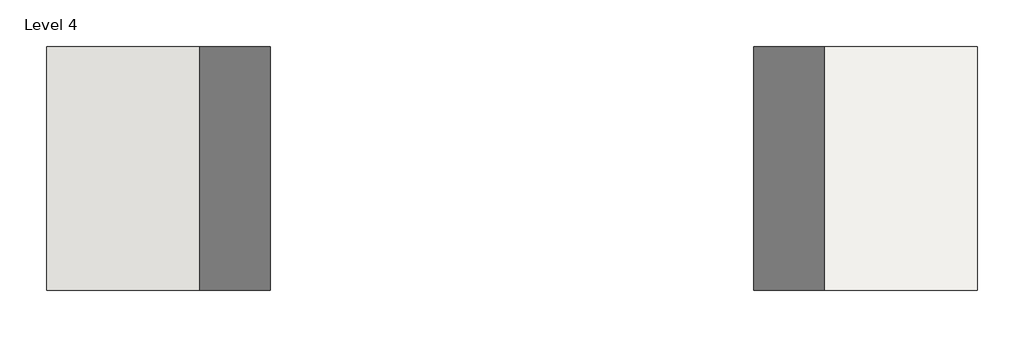
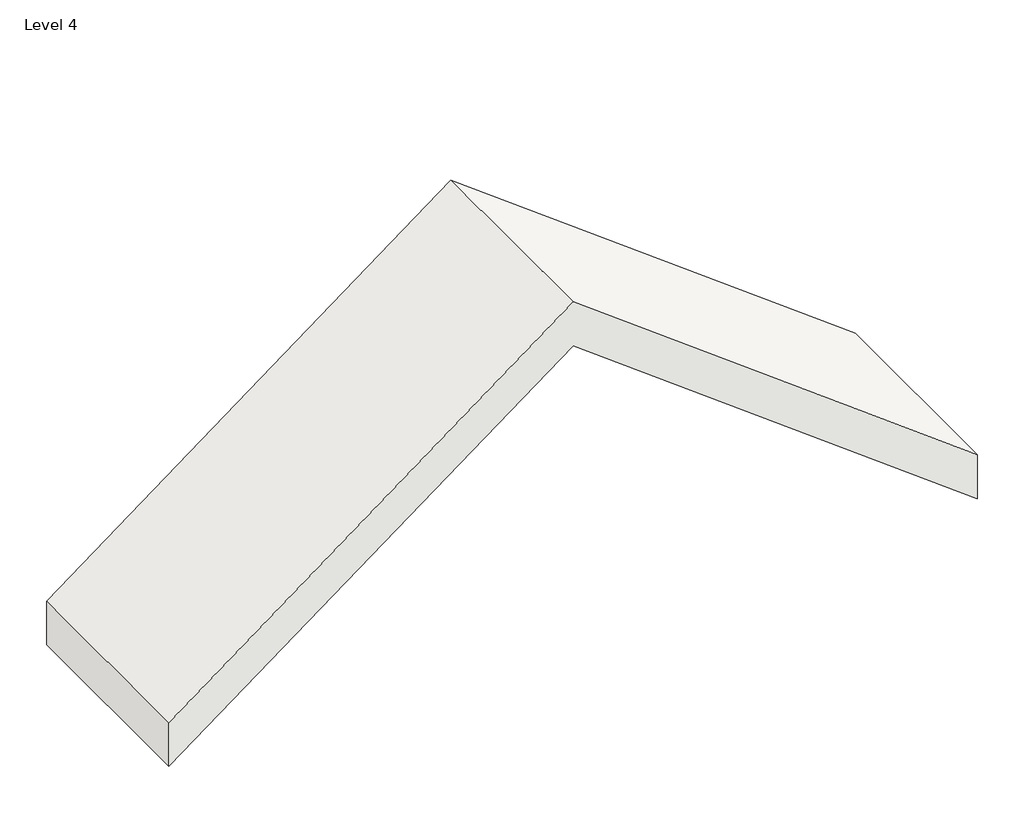
# One storey: 1 roof.
"""IFC4 building model written with IfcOpenShell, lengths in millimetres."""

from ifc_helpers import new_model, si_unit, frame, origin, place, context, project, spatial, polyline, outline, extrude, element, save

model = new_model("IFC4")

# Units and contexts
model_context = context("Model", 3, world=origin())
ifc_project = project(units=[si_unit("LENGTHUNIT", "METRE", prefix="MILLI")], contexts=[model_context])

# Site, building, storey
site = spatial("IfcSite", under=ifc_project)
building = spatial("IfcBuilding", under=site)
storey = spatial("IfcBuildingStorey", under=building, Name="Level 4", Elevation=9144.0)

# Roof
placement = place(None, origin())
element("IfcRoof", 1, ObjectType="Generic - 12\"", at=placement, inside=storey, context=model_context, shape_type="SweptSolid", body=[
    extrude(outline(polyline([(9525.0, -8277.7728383), (12021.7315987, -11606.7483033), (9525.0, -14935.7237683), (9144.0, -14935.7237683), (11640.7315987, -11606.7483033), (9144.0, -8277.7728383), (9525.0, -8277.7728383)])), frame((0.0, -14904.2171312, 0.0), z_axis=(0.0, 1.0, 0.0), x_axis=(0.0, 0.0, 1.0)), (0.0, 0.0, 1.0), 1743.6976162),
])

save(model, "model.ifc")

# Revit data of these elements
# Type "Generic - 12\""
#   Assembly Code = "B1020"
#   Layers, outside or top first: 1' - 0" no material (function 1)
# Element 1 (IfcRoof, "Generic - 12\"")
#   built-in parameter 1001705 = 39.4414 (stored number, unit not read)
#   built-in parameter 1001710 = 33615
#   Phase Created = New Construction
#   Materials on its faces: "Default Roof"
# Materials
#   "Default Roof": colour RGB 88 101 114, transparency 0, Cost = 0
